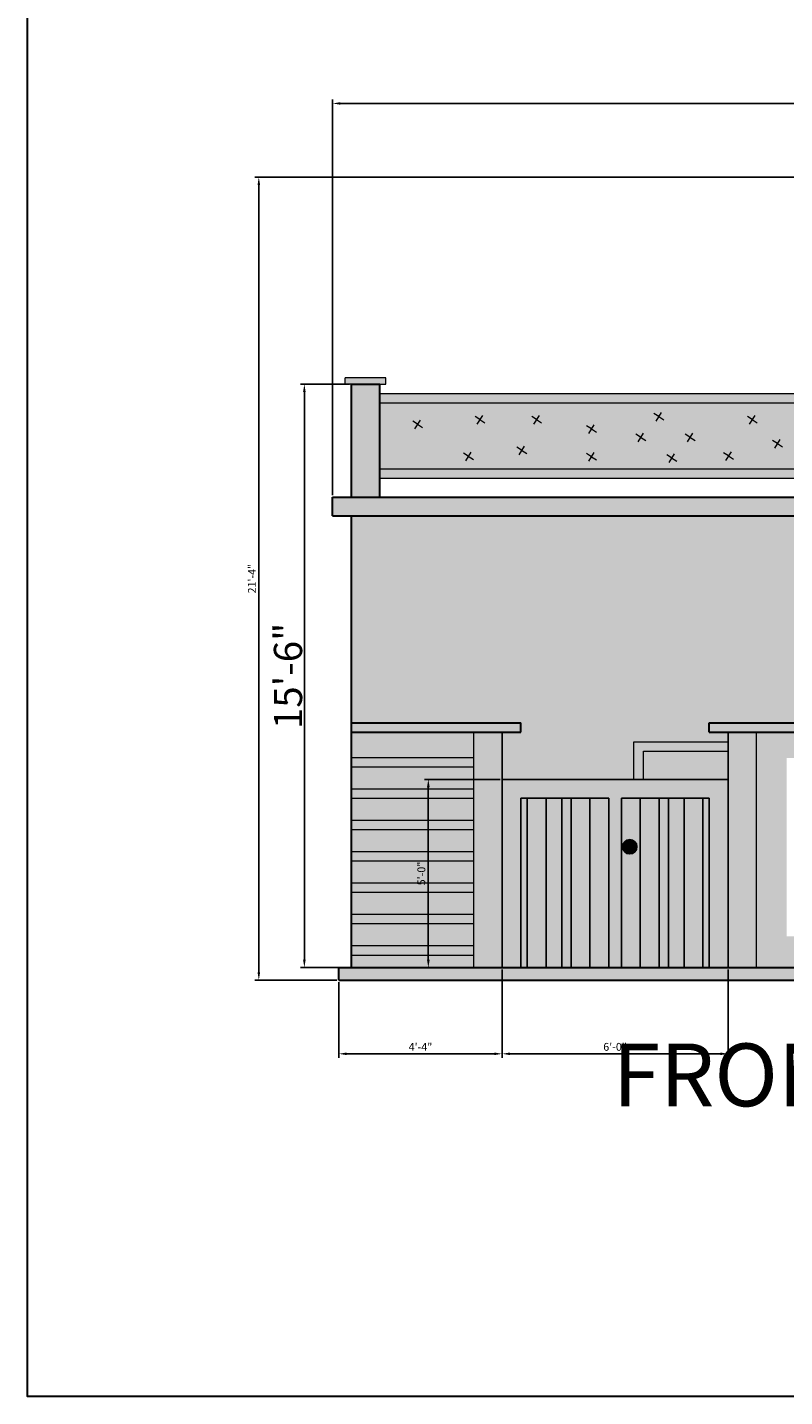
# Model space of a CAD drawing. Units: inches. Extents: x 2163 to 7246, y 928 to 2098.
# Tile 1 of 15: x 2163 to 2404, y 928 to 1365. Entities that reach past the tile are written whole.
import ezdxf

# ---------------------------------------------------------------- set-up
doc = ezdxf.new("R2010")
doc.units = ezdxf.units.IN
for name, color, linetype, lineweight in [('A-ANNO-DIMS', 4, 'Continuous', 18), ('A-ANNO-TITL', 4, 'Continuous', 30), ('A-ANNO-TTLB', 7, 'Continuous', 30), ('A-DOOR', 4, 'Continuous', 25), ('A-DOOR-PATT', 35, 'Continuous', 9), ('A-ELEV', 7, 'Continuous', 30), ('A-ELEV-DETL', 7, 'Continuous', 18)]:
    doc.layers.add(name, color=color, linetype=linetype, lineweight=lineweight)
for name, color, linetype, lineweight, true_color in [('A-ELEV-PATT', 254, 'Continuous', 9, 0xd7ebd2), ('A-ELEV-TRIM-PATT', 11, 'Continuous', 9, 0xf27172), ('A-GLAZ-PATT', 141, 'Continuous', 9, 0xadddf7)]:
    doc.layers.add(name, color=color, linetype=linetype, lineweight=lineweight, true_color=true_color)
doc.styles.get("Standard").update_dxf_attribs({"font": 'arial.ttf'})
doc.dimstyles.new('ISO-25', dxfattribs={"dimtxt": 2.5, "dimasz": 2.5, "dimexe": 1.25, "dimexo": 0.625, "dimtad": 1, "dimdec": 0, "dimlunit": 3, "dimtxsty": 'Standard', "dimcen": 2.5, "dimadec": 0, "dimazin": 0, "dimtfac": 1, "dimtdec": 0, "dimtmove": 0, "dimatfit": 3, "dimfxl": 1, "dimarcsym": 0})

# ---------------------------------------------------------------- blocks, each defined once
blk = doc.blocks.new('*D26')
at = {"layer": 'A-ANNO-DIMS', "color": 0, "lineweight": -2, "transparency": 16777216}
for p, q in [((2265.22, 1251.27), (2249.6, 1251.27)), ((2250.85, 1248.77), (2250.85, 1067.77)), ((2265.22, 1065.27), (2249.6, 1065.27))]:
    blk.add_line(p, q, dxfattribs=at)
at = {"layer": 'A-ANNO-DIMS', "color": 0, "transparency": 16777216}
for points in [[(2250.43, 1248.77), (2251.27, 1248.77), (2250.85, 1251.27)], [(2250.43, 1067.77), (2251.27, 1067.77), (2250.85, 1065.27)]]:
    blk.add_solid(points, dxfattribs=at)
at = {"layer": 'Defpoints', "color": 0, "transparency": 16777216}
for p in [(2265.84, 1251.27), (2250.85, 1065.27), (2265.84, 1065.27)]:
    blk.add_point(p, dxfattribs=at)
at = {"layer": 'A-ANNO-DIMS', "color": 0, "transparency": 16777216, "insert": (2245.63, 1158.27), "char_height": 2.5, "attachment_point": 5, "rotation": 90}
blk.add_mtext('{\\H3.6x;15\'-6"}', dxfattribs=at)
blk = doc.blocks.new('GLASS-PANEL-FITTING')
for p, q in [((1.52, 1.46), (0, 2.43)), ((2.35, 2.77), (0.6, 0)), ((1.52, 1.46), (3.15, 0.44))]:
    blk.add_line(p, q)
blk = doc.blocks.new('*D93')
at = {"layer": 'A-ANNO-DIMS', "color": 0, "lineweight": -2, "transparency": 16777216}
for p, q in [((2259.84, 1215.9), (2259.84, 1342.02)), ((2262.34, 1340.77), (2689.34, 1340.77)), ((2691.84, 1215.9), (2691.84, 1342.02))]:
    blk.add_line(p, q, dxfattribs=at)
at = {"layer": 'A-ANNO-DIMS', "color": 0, "transparency": 16777216}
for points in [[(2262.34, 1341.19), (2262.34, 1340.36), (2259.84, 1340.77)], [(2689.34, 1341.19), (2689.34, 1340.36), (2691.84, 1340.77)]]:
    blk.add_solid(points, dxfattribs=at)
at = {"layer": 'Defpoints', "color": 0, "transparency": 16777216}
for p in [(2691.84, 1340.77), (2259.84, 1215.27), (2691.84, 1215.27)]:
    blk.add_point(p, dxfattribs=at)
at = {"layer": 'A-ANNO-DIMS', "color": 0, "transparency": 16777216, "insert": (2475.84, 1342.68), "char_height": 2.5, "attachment_point": 5}
blk.add_mtext('36\'-0"', dxfattribs=at)
blk = doc.blocks.new('*D94')
at = {"layer": 'A-ANNO-DIMS', "color": 0, "lineweight": -2, "transparency": 16777216}
for p, q in [((2418.22, 1317.27), (2235.09, 1317.27)), ((2236.34, 1314.77), (2236.34, 1063.77)), ((2261.22, 1061.27), (2235.09, 1061.27))]:
    blk.add_line(p, q, dxfattribs=at)
at = {"layer": 'A-ANNO-DIMS', "color": 0, "transparency": 16777216}
for points in [[(2235.93, 1314.77), (2236.76, 1314.77), (2236.34, 1317.27)], [(2235.93, 1063.77), (2236.76, 1063.77), (2236.34, 1061.27)]]:
    blk.add_solid(points, dxfattribs=at)
at = {"layer": 'Defpoints', "color": 0, "transparency": 16777216}
for p in [(2418.84, 1317.27), (2236.34, 1061.27), (2261.84, 1061.27)]:
    blk.add_point(p, dxfattribs=at)
at = {"layer": 'A-ANNO-DIMS', "color": 0, "transparency": 16777216, "insert": (2234.46, 1189.27), "char_height": 2.5, "attachment_point": 5, "rotation": 90}
blk.add_mtext('21\'-4"', dxfattribs=at)
blk = doc.blocks.new('*D96')
at = {"layer": 'A-ANNO-DIMS', "color": 0, "lineweight": -2, "transparency": 16777216}
for p, q in [((2313.84, 1064.65), (2313.84, 1036.52)), ((2261.84, 1060.65), (2261.84, 1036.52)), ((2264.34, 1037.77), (2311.34, 1037.77))]:
    blk.add_line(p, q, dxfattribs=at)
at = {"layer": 'A-ANNO-DIMS', "color": 0, "transparency": 16777216}
for points in [[(2264.34, 1038.19), (2264.34, 1037.36), (2261.84, 1037.77)], [(2311.34, 1038.19), (2311.34, 1037.36), (2313.84, 1037.77)]]:
    blk.add_solid(points, dxfattribs=at)
at = {"layer": 'Defpoints', "color": 0, "transparency": 16777216}
for p in [(2313.84, 1065.27), (2261.84, 1061.27), (2313.84, 1037.77)]:
    blk.add_point(p, dxfattribs=at)
at = {"layer": 'A-ANNO-DIMS', "color": 0, "transparency": 16777216, "insert": (2287.84, 1039.65), "char_height": 2.5, "attachment_point": 5}
blk.add_mtext('4\'-4"', dxfattribs=at)
blk = doc.blocks.new('*D97')
at = {"layer": 'A-ANNO-DIMS', "color": 0, "lineweight": -2, "transparency": 16777216}
for p, q in [((2313.84, 1064.65), (2313.84, 1036.52)), ((2385.84, 1064.65), (2385.84, 1036.52)), ((2316.34, 1037.77), (2383.34, 1037.77))]:
    blk.add_line(p, q, dxfattribs=at)
at = {"layer": 'A-ANNO-DIMS', "color": 0, "transparency": 16777216}
for points in [[(2316.34, 1038.19), (2316.34, 1037.36), (2313.84, 1037.77)], [(2383.34, 1038.19), (2383.34, 1037.36), (2385.84, 1037.77)]]:
    blk.add_solid(points, dxfattribs=at)
at = {"layer": 'Defpoints', "color": 0, "transparency": 16777216}
for p in [(2313.84, 1065.27), (2385.84, 1065.27), (2385.84, 1037.77)]:
    blk.add_point(p, dxfattribs=at)
at = {"layer": 'A-ANNO-DIMS', "color": 0, "transparency": 16777216, "insert": (2349.84, 1039.67), "char_height": 2.5, "attachment_point": 5}
blk.add_mtext('6\'-0"', dxfattribs=at)
blk = doc.blocks.new('*D98')
at = {"layer": 'A-ANNO-DIMS', "color": 0, "lineweight": -2, "transparency": 16777216}
for p, q in [((2313.22, 1125.27), (2289.09, 1125.27)), ((2290.34, 1067.77), (2290.34, 1122.77)), ((2313.22, 1065.27), (2289.09, 1065.27))]:
    blk.add_line(p, q, dxfattribs=at)
at = {"layer": 'A-ANNO-DIMS', "color": 0, "transparency": 16777216}
for points in [[(2289.93, 1122.77), (2290.76, 1122.77), (2290.34, 1125.27)], [(2289.93, 1067.77), (2290.76, 1067.77), (2290.34, 1065.27)]]:
    blk.add_solid(points, dxfattribs=at)
at = {"layer": 'Defpoints', "color": 0, "transparency": 16777216}
for p in [(2290.34, 1125.27), (2313.84, 1125.27), (2313.84, 1065.27)]:
    blk.add_point(p, dxfattribs=at)
at = {"layer": 'A-ANNO-DIMS', "color": 0, "transparency": 16777216, "insert": (2288.44, 1095.27), "char_height": 2.5, "attachment_point": 5, "rotation": 90}
blk.add_mtext('5\'-0"', dxfattribs=at)

msp = doc.modelspace()

# ---------------------------------------------------------------- hatches: boundary and pattern name
at = {"layer": 'A-DOOR-PATT'}
h = msp.add_hatch(color=256, dxfattribs=at)
h.dxf.hatch_style = 1
h.paths.add_polyline_path([(2357.84, 1119.27), (2351.84, 1119.27), (2351.84, 1065.27), (2357.84, 1065.27)], flags=17)
h.paths.add_polyline_path([(2356.8, 1103.78, -1), (2352.24, 1103.78, -1)], flags=16)
h.paths.add_polyline_path([(2355.92, 1103.78, -1), (2353.13, 1103.78, -1)], flags=0)
h.paths.add_polyline_path([(2377.84, 1119.27), (2371.84, 1119.27), (2371.84, 1065.27), (2377.84, 1065.27)], flags=17)
h.paths.add_polyline_path([(2379.84, 1065.27), (2385.84, 1065.27), (2385.84, 1125.27), (2313.84, 1125.27), (2313.84, 1065.27), (2319.84, 1065.27), (2319.84, 1119.27), (2347.84, 1119.27), (2347.84, 1065.27), (2351.84, 1065.27), (2351.84, 1119.27), (2379.84, 1119.27)])
h.paths.add_polyline_path([(2327.84, 1119.27), (2321.84, 1119.27), (2321.84, 1065.27), (2327.84, 1065.27)], flags=17)
h.paths.add_polyline_path([(2341.84, 1065.27), (2347.84, 1065.27), (2347.84, 1119.27), (2341.84, 1119.27)], flags=17)
h = msp.add_hatch(color=256, dxfattribs=at)
h.dxf.hatch_style = 1
h.paths.add_polyline_path([(2319.84, 1065.27), (2321.84, 1065.27), (2321.84, 1119.27), (2319.84, 1119.27)])
h.paths.add_polyline_path([(2377.84, 1065.27), (2379.84, 1065.27), (2379.84, 1119.27), (2377.84, 1119.27)])
h = msp.add_hatch(color=256, dxfattribs=at)
h.dxf.hatch_style = 1
h.paths.add_polyline_path([(2371.84, 1119.27), (2366.84, 1119.27), (2366.84, 1065.27), (2371.84, 1065.27)])
h.paths.add_polyline_path([(2363.84, 1119.27), (2357.84, 1119.27), (2357.84, 1065.27), (2363.84, 1065.27)])
h.paths.add_polyline_path([(2341.84, 1119.27), (2335.84, 1119.27), (2335.84, 1065.27), (2341.84, 1065.27)])
h.paths.add_polyline_path([(2332.84, 1119.27), (2327.84, 1119.27), (2327.84, 1065.27), (2332.84, 1065.27)])
h = msp.add_hatch(color=256, dxfattribs=at)
h.dxf.hatch_style = 1
h.paths.add_polyline_path([(2332.84, 1065.27), (2335.84, 1065.27), (2335.84, 1119.27), (2332.84, 1119.27)])
h.paths.add_polyline_path([(2366.84, 1119.27), (2363.84, 1119.27), (2363.84, 1065.27), (2366.84, 1065.27)])
h = msp.add_hatch(color=256, dxfattribs=at)
h.dxf.hatch_style = 1
h.paths.add_polyline_path([(2356.8, 1103.78, 1), (2352.24, 1103.78, 1)])
h.paths.add_polyline_path([(2355.92, 1103.78, 1), (2353.13, 1103.78, 1)], flags=16)
h = msp.add_hatch(color=256, dxfattribs=at)
h.dxf.hatch_style = 1
h.paths.add_polyline_path([(2355.92, 1103.78, 1), (2353.13, 1103.78, 1)])
at = {"layer": 'A-ELEV-PATT'}
h = msp.add_hatch(color=256, dxfattribs=at)
h.dxf.hatch_style = 1
h.paths.add_polyline_path([(2274.84, 1251.27), (2265.84, 1251.27), (2265.84, 1215.27), (2274.84, 1215.27)])
h = msp.add_hatch(color=256, dxfattribs=at)
h.dxf.hatch_style = 1
h.paths.add_polyline_path([(2436.84, 1209.27), (2265.84, 1209.27), (2265.84, 1143.27), (2319.84, 1143.27), (2319.84, 1140.27), (2313.84, 1140.27), (2313.84, 1125.27), (2355.84, 1125.27), (2355.84, 1137.27), (2385.84, 1137.27), (2385.84, 1140.27), (2379.84, 1140.27), (2379.84, 1143.27), (2436.84, 1143.27)])
h.paths.add_polyline_path([(2676.84, 1209.27), (2536.84, 1209.27), (2536.84, 1143.27), (2676.84, 1143.27)])
h = msp.add_hatch(color=256, dxfattribs=at)
h.dxf.hatch_style = 1
h.paths.add_polyline_path([(2265.84, 1140.27), (2265.84, 1132.27), (2304.84, 1132.27), (2304.84, 1140.27)])
h.paths.add_polyline_path([(2304.84, 1122.27), (2304.84, 1129.27), (2265.84, 1129.27), (2265.84, 1122.27)])
h.paths.add_polyline_path([(2265.84, 1119.27), (2265.84, 1112.27), (2304.84, 1112.27), (2304.84, 1119.27)])
h.paths.add_polyline_path([(2304.84, 1102.27), (2304.84, 1109.27), (2265.84, 1109.27), (2265.84, 1102.27)])
h.paths.add_polyline_path([(2304.84, 1092.27), (2304.84, 1099.27), (2265.84, 1099.27), (2265.84, 1092.27)])
h.paths.add_polyline_path([(2265.84, 1089.27), (2265.84, 1082.27), (2304.84, 1082.27), (2304.84, 1089.27)])
h.paths.add_polyline_path([(2265.84, 1079.27), (2265.84, 1072.27), (2304.84, 1072.27), (2304.84, 1079.27)])
h.paths.add_polyline_path([(2265.84, 1069.27), (2265.84, 1065.27), (2304.84, 1065.27), (2304.84, 1069.27)])
h = msp.add_hatch(color=256, dxfattribs=at)
h.dxf.hatch_style = 1
h.paths.add_polyline_path([(2313.84, 1140.27), (2304.84, 1140.27), (2304.84, 1065.27), (2313.84, 1065.27)])
h.paths.add_polyline_path([(2394.84, 1140.27), (2385.84, 1140.27), (2385.84, 1065.27), (2394.84, 1065.27)])
h = msp.add_hatch(color=256, dxfattribs=at)
h.dxf.hatch_style = 1
h.paths.add_polyline_path([(2672.86, 1078.23), (2672.86, 1129.07), (2407.51, 1129.07), (2407.51, 1078.23)], flags=0)
h.paths.add_polyline_path([(2447.87, 1100.37, -1), (2480.27, 1100.37, -1)], flags=0)
h.paths.add_polyline_path([(2429.94, 1087.24, -1), (2415.68, 1087.24, -1)], flags=0)
h.paths.add_polyline_path([(2414.43, 1113.86, -1), (2434.12, 1113.86, -1)], flags=0)
h.paths.add_polyline_path([(2498.1, 1111.99, -1), (2524.62, 1111.99, -1)], flags=0)
h.paths.add_polyline_path([(2513.98, 1085.52, -1), (2502.02, 1085.52, -1)], flags=0)
h.paths.add_polyline_path([(2583.51, 1102.62, -1), (2544.32, 1102.62, -1)], flags=0)
h.paths.add_polyline_path([(2621.72, 1099.62, -1), (2603.71, 1099.62, -1)], flags=0)
h.paths.add_polyline_path([(2666.17, 1104.49, -1), (2630.59, 1104.49, -1)], flags=0)
h.paths.add_polyline_path([(2394.84, 1065.27), (2685.84, 1065.27), (2685.84, 1140.27), (2676.84, 1140.27), (2394.84, 1140.27)])
h.paths.add_polyline_path([(2404.51, 1132.07), (2675.86, 1132.07), (2675.86, 1075.23), (2404.51, 1075.23)], flags=16)
h.paths.add_polyline_path([(2407.51, 1129.07), (2672.86, 1129.07), (2672.86, 1078.23), (2407.51, 1078.23)], flags=0)
h = msp.add_hatch(color=256, dxfattribs=at)
h.dxf.hatch_style = 1
h.paths.add_polyline_path([(2265.84, 1132.27), (2265.84, 1129.27), (2304.84, 1129.27), (2304.84, 1132.27)])
h.paths.add_polyline_path([(2304.84, 1119.27), (2304.84, 1122.27), (2265.84, 1122.27), (2265.84, 1119.27)])
h.paths.add_polyline_path([(2304.84, 1109.27), (2304.84, 1112.27), (2265.84, 1112.27), (2265.84, 1109.27)])
h.paths.add_polyline_path([(2304.84, 1099.27), (2304.84, 1102.27), (2265.84, 1102.27), (2265.84, 1099.27)])
h = msp.add_hatch(color=256, dxfattribs=at)
h.dxf.hatch_style = 1
h.paths.add_polyline_path([(2304.84, 1069.27), (2304.84, 1072.27), (2265.84, 1072.27), (2265.84, 1069.27)])
h.paths.add_polyline_path([(2265.84, 1082.27), (2265.84, 1079.27), (2304.84, 1079.27), (2304.84, 1082.27)])
h.paths.add_polyline_path([(2304.84, 1089.27), (2304.84, 1092.27), (2265.84, 1092.27), (2265.84, 1089.27)])
at = {"layer": 'A-ELEV-TRIM-PATT'}
h = msp.add_hatch(color=256, dxfattribs=at)
h.dxf.hatch_style = 1
h.paths.add_polyline_path([(2276.84, 1253.27), (2263.84, 1253.27), (2263.84, 1251.27), (2265.84, 1251.27), (2274.84, 1251.27), (2276.84, 1251.27)])
h.paths.add_polyline_path([(2687.84, 1253.27), (2676.84, 1253.27), (2674.84, 1253.27), (2674.84, 1251.27), (2676.84, 1251.27), (2685.84, 1251.27), (2687.84, 1251.27)])
h = msp.add_hatch(color=256, dxfattribs=at)
h.dxf.hatch_style = 1
h.paths.add_polyline_path([(2436.84, 1248.27), (2274.84, 1248.27), (2274.84, 1245.27), (2436.84, 1245.27)])
h.paths.add_polyline_path([(2436.84, 1224.27), (2274.84, 1224.27), (2274.84, 1221.27), (2436.84, 1221.27)])
h.paths.add_polyline_path([(2676.84, 1248.27), (2536.84, 1248.27), (2536.84, 1245.27), (2676.84, 1245.27)])
h.paths.add_polyline_path([(2676.84, 1224.27), (2536.84, 1224.27), (2536.84, 1221.27), (2676.84, 1221.27)])
h = msp.add_hatch(color=256, dxfattribs=at)
h.dxf.hatch_style = 1
h.paths.add_polyline_path([(2536.84, 1215.27), (2536.84, 1209.27), (2691.84, 1209.27), (2691.84, 1215.27)])
h.paths.add_polyline_path([(2259.84, 1215.27), (2259.84, 1209.27), (2436.84, 1209.27), (2436.84, 1215.27)])
h = msp.add_hatch(color=256, dxfattribs=at)
h.dxf.hatch_style = 1
h.paths.add_polyline_path([(2319.84, 1143.27), (2265.84, 1143.27), (2265.84, 1140.27), (2319.84, 1140.27)])
h.paths.add_polyline_path([(2676.84, 1143.27), (2379.84, 1143.27), (2379.84, 1140.27), (2676.84, 1140.27)])
h = msp.add_hatch(color=256, dxfattribs=at)
h.dxf.hatch_style = 1
h.paths.add_polyline_path([(2685.84, 1140.27), (2685.84, 1143.27), (2676.84, 1143.27), (2379.84, 1143.27), (2379.84, 1140.27), (2676.84, 1140.27)])
h = msp.add_hatch(color=256, dxfattribs=at)
h.dxf.hatch_style = 1
h.paths.add_polyline_path([(2385.84, 1134.27), (2385.84, 1137.27), (2355.84, 1137.27), (2355.84, 1125.27), (2358.84, 1125.27), (2358.84, 1134.27)])
h = msp.add_hatch(color=256, dxfattribs=at)
h.dxf.hatch_style = 1
h.paths.add_polyline_path([(2689.84, 1061.27), (2689.84, 1065.27), (2261.84, 1065.27), (2261.84, 1061.27)])
at = {"layer": 'A-GLAZ-PATT'}
h = msp.add_hatch(color=256, dxfattribs=at)
h.dxf.hatch_style = 1
h.paths.add_polyline_path([(2436.84, 1224.27), (2436.84, 1245.27), (2274.84, 1245.27), (2274.84, 1224.27)])
h.paths.add_polyline_path([(2536.84, 1245.27), (2536.84, 1224.27), (2676.84, 1224.27), (2676.84, 1245.27)])
h = msp.add_hatch(color=256, dxfattribs=at)
h.dxf.hatch_style = 1
h.paths.add_polyline_path([(2358.84, 1134.27), (2358.84, 1125.27), (2385.84, 1125.27), (2385.84, 1134.27)])

# ---------------------------------------------------------------- linework, layer by layer
at = {"layer": 'A-ANNO-TTLB'}
msp.add_lwpolyline([(2162.62, 2098.21), (3633.38, 2098.21), (3633.38, 928.48), (2162.62, 928.48)], close=True, dxfattribs=at)
at = {"layer": 'A-DOOR'}
for p, q in [((2313.84, 1065.27), (2313.84, 1140.27)), ((2385.84, 1065.27), (2385.84, 1140.27)), ((2313.84, 1125.27), (2385.84, 1125.27)), ((2319.84, 1065.27), (2319.84, 1119.27)), ((2319.84, 1119.27), (2347.84, 1119.27)), ((2321.84, 1065.27), (2321.84, 1119.27)), ((2327.84, 1065.27), (2327.84, 1119.27)), ((2332.84, 1119.27), (2332.84, 1065.27)), ((2335.84, 1119.27), (2335.84, 1065.27)), ((2341.84, 1119.27), (2341.84, 1065.27)), ((2347.84, 1119.27), (2347.84, 1065.27)), ((2351.84, 1119.27), (2351.84, 1065.27)), ((2351.84, 1119.27), (2379.84, 1119.27)), ((2357.84, 1119.27), (2357.84, 1065.27)), ((2363.84, 1119.27), (2363.84, 1065.27)), ((2366.84, 1119.27), (2366.84, 1065.27)), ((2371.84, 1065.27), (2371.84, 1119.27)), ((2377.84, 1065.27), (2377.84, 1119.27)), ((2379.84, 1065.27), (2379.84, 1119.27))]:
    msp.add_line(p, q, dxfattribs=at)
for radius in [2.28, 1.4]:
    msp.add_circle((2354.52, 1103.78), radius, dxfattribs=at)
at = {"layer": 'A-ELEV'}
for p, q in [((2265.84, 1251.27), (2274.84, 1251.27)), ((2265.84, 1215.27), (2265.84, 1251.27)), ((2274.84, 1215.27), (2274.84, 1251.27)), ((2259.84, 1215.27), (2436.84, 1215.27)), ((2259.84, 1209.27), (2259.84, 1215.27)), ((2259.84, 1209.27), (2436.84, 1209.27)), ((2265.84, 1065.27), (2265.84, 1209.27)), ((2265.84, 1143.27), (2319.84, 1143.27)), ((2265.84, 1140.27), (2319.84, 1140.27)), ((2319.84, 1140.27), (2319.84, 1143.27)), ((2379.84, 1143.27), (2676.84, 1143.27)), ((2379.84, 1140.27), (2379.84, 1143.27)), ((2379.84, 1140.27), (2676.84, 1140.27)), ((2261.84, 1065.27), (2689.84, 1065.27)), ((2261.84, 1061.27), (2261.84, 1065.27)), ((2261.84, 1061.27), (2689.84, 1061.27))]:
    msp.add_line(p, q, dxfattribs=at)
at = {"layer": 'A-ELEV-DETL'}
for p, q in [((2263.84, 1251.27), (2263.84, 1253.27)), ((2276.84, 1253.27), (2263.84, 1253.27)), ((2276.84, 1251.27), (2276.84, 1253.27)), ((2265.84, 1251.27), (2263.84, 1251.27)), ((2274.84, 1251.27), (2265.84, 1251.27)), ((2265.84, 1251.27), (2265.84, 1215.27)), ((2274.84, 1251.27), (2276.84, 1251.27)), ((2274.84, 1215.27), (2274.84, 1251.27)), ((2274.84, 1248.27), (2436.84, 1248.27)), ((2274.84, 1245.27), (2436.84, 1245.27)), ((2274.84, 1224.27), (2436.84, 1224.27)), ((2274.84, 1221.27), (2436.84, 1221.27)), ((2265.84, 1215.27), (2274.84, 1215.27)), ((2304.84, 1065.27), (2304.84, 1140.27)), ((2394.84, 1065.27), (2394.84, 1140.27)), ((2355.84, 1125.27), (2355.84, 1137.27)), ((2355.84, 1137.27), (2385.84, 1137.27)), ((2265.84, 1132.27), (2304.84, 1132.27)), ((2358.84, 1125.27), (2358.84, 1134.27)), ((2358.84, 1134.27), (2385.84, 1134.27)), ((2265.84, 1129.27), (2304.84, 1129.27)), ((2265.84, 1122.27), (2304.84, 1122.27)), ((2265.84, 1119.27), (2304.84, 1119.27)), ((2265.84, 1112.27), (2304.84, 1112.27)), ((2265.84, 1109.27), (2304.84, 1109.27)), ((2265.84, 1102.27), (2304.84, 1102.27)), ((2265.84, 1099.27), (2304.84, 1099.27)), ((2265.84, 1092.27), (2304.84, 1092.27)), ((2265.84, 1089.27), (2304.84, 1089.27)), ((2265.84, 1082.27), (2304.84, 1082.27)), ((2265.84, 1079.27), (2304.84, 1079.27)), ((2265.84, 1072.27), (2304.84, 1072.27)), ((2265.84, 1069.27), (2304.84, 1069.27))]:
    msp.add_line(p, q, dxfattribs=at)

# ---------------------------------------------------------------- block references
for p in [(2285.38, 1237.05), (2305.22, 1238.53), (2323.29, 1238.53), (2362.22, 1239.51), (2391.99, 1238.53), (2340.76, 1235.57), (2356.45, 1232.91), (2372.15, 1232.91), (2318.55, 1228.76), (2400.01, 1230.87), (2301.56, 1226.84), (2340.76, 1226.69), (2366.31, 1226.32), (2384.43, 1226.92)]:
    msp.add_blockref('GLASS-PANEL-FITTING', p, dxfattribs=at)

# ---------------------------------------------------------------- texts
at = {"layer": 'A-ANNO-TITL', "insert": (2349.09, 1041.06), "char_height": 20, "attachment_point": 1}
msp.add_mtext_dynamic_manual_height_columns('FRONT ELEVATION', width=571.2399, gutter_width=12.5, heights=[0], dxfattribs=at)

# ---------------------------------------------------------------- dimensions: what is measured, and where the dimension line sits
at = {"layer": 'A-ANNO-DIMS'}
for base, p1, p2, picture, middle in [((2691.84, 1340.77), (2259.84, 1215.27), (2691.84, 1215.27), '*D93', (2475.84, 1342.68)), ((2313.84, 1037.77), (2261.84, 1061.27), (2313.84, 1065.27), '*D96', (2287.84, 1039.65)), ((2385.84, 1037.77), (2313.84, 1065.27), (2385.84, 1065.27), '*D97', (2349.84, 1039.67))]:
    dim = msp.add_linear_dim(base=base, p1=p1, p2=p2, dimstyle='ISO-25', override={"dimdec": 1, "dimlfac": 1, "dimrnd": 0, "dimzin": 1, "dimdsep": 46, "dimlunit": 4, "dimfrac": 2}, dxfattribs=at)
    dim.commit()
    dim.dimension.update_dxf_attribs({"geometry": picture, "text_midpoint": middle})
for base, p1, p2, picture, middle in [((2236.34, 1061.27), (2418.84, 1317.27), (2261.84, 1061.27), '*D94', (2234.46, 1189.27)), ((2290.34, 1125.27), (2313.84, 1065.27), (2313.84, 1125.27), '*D98', (2288.44, 1095.27))]:
    dim = msp.add_linear_dim(base=base, p1=p1, p2=p2, angle=90, dimstyle='ISO-25', override={"dimdec": 1, "dimlfac": 1, "dimrnd": 0, "dimzin": 1, "dimdsep": 46, "dimlunit": 4, "dimfrac": 2}, dxfattribs=at)
    dim.commit()
    dim.dimension.update_dxf_attribs({"geometry": picture, "text_midpoint": middle})
dim = msp.add_linear_dim(base=(2250.85, 1065.27), p1=(2265.84, 1251.27), p2=(2265.84, 1065.27), angle=90, text='{\\H3.6x;<>}', dimstyle='ISO-25', override={"dimclrd": 0, "dimclre": 0, "dimclrt": 0}, dxfattribs=at)
dim.commit()
dim.dimension.update_dxf_attribs({"geometry": '*D26', "text_midpoint": (2245.63, 1158.27)})

doc.saveas('drawing.dxf')
